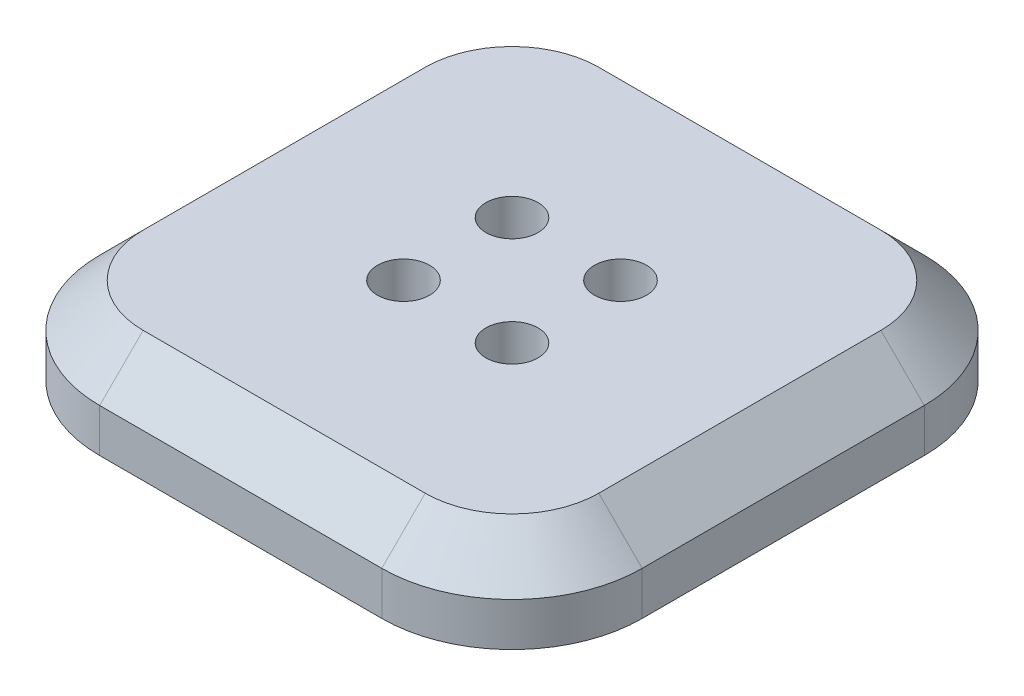
ISO-10303-21;
HEADER;
FILE_DESCRIPTION(('STEP AP214'),'2;1');
FILE_NAME('part.step','',(''),(''),'','','');
FILE_SCHEMA(('AUTOMOTIVE_DESIGN { 1 0 10303 214 1 1 1 1 }'));
ENDSEC;
DATA;
#1=APPLICATION_CONTEXT('core data for automotive mechanical design processes');
#2=APPLICATION_PROTOCOL_DEFINITION('international standard','automotive_design',2000,#1);
#3=PRODUCT_CONTEXT('',#1,'mechanical');
#4=PRODUCT('Part','Part','',(#3));
#5=PRODUCT_RELATED_PRODUCT_CATEGORY('part','',(#4));
#6=PRODUCT_DEFINITION_FORMATION('','',#4);
#7=PRODUCT_DEFINITION_CONTEXT('part definition',#1,'design');
#8=PRODUCT_DEFINITION('design','',#6,#7);
#9=PRODUCT_DEFINITION_SHAPE('','',#8);
#10=(LENGTH_UNIT() NAMED_UNIT(*) SI_UNIT(.MILLI.,.METRE.));
#11=(NAMED_UNIT(*) PLANE_ANGLE_UNIT() SI_UNIT($,.RADIAN.));
#12=(NAMED_UNIT(*) SI_UNIT($,.STERADIAN.) SOLID_ANGLE_UNIT());
#13=UNCERTAINTY_MEASURE_WITH_UNIT(LENGTH_MEASURE(1.E-05),#10,'distance_accuracy_value','');
#14=(GEOMETRIC_REPRESENTATION_CONTEXT(3) GLOBAL_UNCERTAINTY_ASSIGNED_CONTEXT((#13)) GLOBAL_UNIT_ASSIGNED_CONTEXT((#10,
#11,#12)) REPRESENTATION_CONTEXT('',''));
#15=CARTESIAN_POINT('',(0.,0.,0.));
#16=DIRECTION('',(0.,0.,1.));
#17=DIRECTION('',(1.,0.,0.));
#18=AXIS2_PLACEMENT_3D('',#15,#16,#17);
#19=CARTESIAN_POINT('',(62.5,20.,62.5));
#20=DIRECTION('',(-1.,0.,0.));
#21=DIRECTION('',(0.,0.,1.));
#22=AXIS2_PLACEMENT_3D('',#19,#20,#21);
#23=PLANE('',#22);
#24=DIRECTION('',(0.,-1.,0.));
#25=VECTOR('',#24,1.);
#26=CARTESIAN_POINT('',(62.5,20.,-32.5));
#27=LINE('',#26,#25);
#28=CARTESIAN_POINT('',(62.5,0.,-32.5));
#29=VERTEX_POINT('',#28);
#30=CARTESIAN_POINT('',(62.5,9.99999999999996,-32.5));
#31=VERTEX_POINT('',#30);
#32=EDGE_CURVE('E242',#29,#31,#27,.F.);
#33=ORIENTED_EDGE('',*,*,#32,.T.);
#34=DIRECTION('',(0.,0.,1.));
#35=VECTOR('',#34,1.);
#36=CARTESIAN_POINT('',(62.5,9.99999999999996,62.5));
#37=LINE('',#36,#35);
#38=CARTESIAN_POINT('',(62.5,9.99999999999996,32.5));
#39=VERTEX_POINT('',#38);
#40=EDGE_CURVE('E11',#31,#39,#37,.T.);
#41=ORIENTED_EDGE('',*,*,#40,.T.);
#42=DIRECTION('',(0.,-1.,0.));
#43=VECTOR('',#42,1.);
#44=CARTESIAN_POINT('',(62.5,20.,32.5));
#45=LINE('',#44,#43);
#46=CARTESIAN_POINT('',(62.5,0.,32.5));
#47=VERTEX_POINT('',#46);
#48=EDGE_CURVE('E245',#39,#47,#45,.T.);
#49=ORIENTED_EDGE('',*,*,#48,.T.);
#50=DIRECTION('',(0.,0.,-1.));
#51=VECTOR('',#50,1.);
#52=CARTESIAN_POINT('',(62.5,0.,62.5));
#53=LINE('',#52,#51);
#54=EDGE_CURVE('E215',#47,#29,#53,.T.);
#55=ORIENTED_EDGE('',*,*,#54,.T.);
#56=EDGE_LOOP('',(#33,#41,#49,#55));
#57=FACE_BOUND('',#56,.T.);
#58=ADVANCED_FACE('F41',(#57),#23,.F.);
#59=CARTESIAN_POINT('',(-62.5,20.,-62.5));
#60=DIRECTION('',(0.,0.,1.));
#61=DIRECTION('',(1.,0.,0.));
#62=AXIS2_PLACEMENT_3D('',#59,#60,#61);
#63=PLANE('',#62);
#64=DIRECTION('',(0.,-1.,0.));
#65=VECTOR('',#64,1.);
#66=CARTESIAN_POINT('',(-32.5,20.,-62.5));
#67=LINE('',#66,#65);
#68=CARTESIAN_POINT('',(-32.5,0.,-62.5));
#69=VERTEX_POINT('',#68);
#70=CARTESIAN_POINT('',(-32.5,9.99999999999996,-62.5));
#71=VERTEX_POINT('',#70);
#72=EDGE_CURVE('E239',#69,#71,#67,.F.);
#73=ORIENTED_EDGE('',*,*,#72,.T.);
#74=DIRECTION('',(1.,0.,0.));
#75=VECTOR('',#74,1.);
#76=CARTESIAN_POINT('',(-62.5,9.99999999999996,-62.5));
#77=LINE('',#76,#75);
#78=CARTESIAN_POINT('',(32.5,9.99999999999996,-62.5));
#79=VERTEX_POINT('',#78);
#80=EDGE_CURVE('E280',#71,#79,#77,.T.);
#81=ORIENTED_EDGE('',*,*,#80,.T.);
#82=DIRECTION('',(0.,-1.,0.));
#83=VECTOR('',#82,1.);
#84=CARTESIAN_POINT('',(32.5,20.,-62.5));
#85=LINE('',#84,#83);
#86=CARTESIAN_POINT('',(32.5,0.,-62.5));
#87=VERTEX_POINT('',#86);
#88=EDGE_CURVE('E240',#79,#87,#85,.T.);
#89=ORIENTED_EDGE('',*,*,#88,.T.);
#90=DIRECTION('',(-1.,0.,0.));
#91=VECTOR('',#90,1.);
#92=CARTESIAN_POINT('',(-62.5,0.,-62.5));
#93=LINE('',#92,#91);
#94=EDGE_CURVE('E214',#87,#69,#93,.T.);
#95=ORIENTED_EDGE('',*,*,#94,.T.);
#96=EDGE_LOOP('',(#73,#81,#89,#95));
#97=FACE_BOUND('',#96,.T.);
#98=ADVANCED_FACE('F335',(#97),#63,.F.);
#99=CARTESIAN_POINT('',(-62.5,20.,62.5));
#100=DIRECTION('',(1.,0.,0.));
#101=DIRECTION('',(0.,0.,-1.));
#102=AXIS2_PLACEMENT_3D('',#99,#100,#101);
#103=PLANE('',#102);
#104=DIRECTION('',(0.,-1.,0.));
#105=VECTOR('',#104,1.);
#106=CARTESIAN_POINT('',(-62.5,20.,32.5));
#107=LINE('',#106,#105);
#108=CARTESIAN_POINT('',(-62.5,0.,32.5));
#109=VERTEX_POINT('',#108);
#110=CARTESIAN_POINT('',(-62.5,9.99999999999996,32.5));
#111=VERTEX_POINT('',#110);
#112=EDGE_CURVE('E221',#109,#111,#107,.F.);
#113=ORIENTED_EDGE('',*,*,#112,.T.);
#114=DIRECTION('',(0.,0.,-1.));
#115=VECTOR('',#114,1.);
#116=CARTESIAN_POINT('',(-62.5,9.99999999999996,62.5));
#117=LINE('',#116,#115);
#118=CARTESIAN_POINT('',(-62.5,9.99999999999996,-32.5));
#119=VERTEX_POINT('',#118);
#120=EDGE_CURVE('E268',#111,#119,#117,.T.);
#121=ORIENTED_EDGE('',*,*,#120,.T.);
#122=DIRECTION('',(0.,-1.,0.));
#123=VECTOR('',#122,1.);
#124=CARTESIAN_POINT('',(-62.5,20.,-32.5));
#125=LINE('',#124,#123);
#126=CARTESIAN_POINT('',(-62.5,0.,-32.5));
#127=VERTEX_POINT('',#126);
#128=EDGE_CURVE('E230',#119,#127,#125,.T.);
#129=ORIENTED_EDGE('',*,*,#128,.T.);
#130=DIRECTION('',(0.,0.,1.));
#131=VECTOR('',#130,1.);
#132=CARTESIAN_POINT('',(-62.5,0.,62.5));
#133=LINE('',#132,#131);
#134=EDGE_CURVE('E217',#127,#109,#133,.T.);
#135=ORIENTED_EDGE('',*,*,#134,.T.);
#136=EDGE_LOOP('',(#113,#121,#129,#135));
#137=FACE_BOUND('',#136,.T.);
#138=ADVANCED_FACE('F347',(#137),#103,.F.);
#139=CARTESIAN_POINT('',(-62.5,20.,62.5));
#140=DIRECTION('',(0.,0.,-1.));
#141=DIRECTION('',(-1.,0.,0.));
#142=AXIS2_PLACEMENT_3D('',#139,#140,#141);
#143=PLANE('',#142);
#144=DIRECTION('',(0.,-1.,0.));
#145=VECTOR('',#144,1.);
#146=CARTESIAN_POINT('',(32.5,20.,62.5));
#147=LINE('',#146,#145);
#148=CARTESIAN_POINT('',(32.5,0.,62.5));
#149=VERTEX_POINT('',#148);
#150=CARTESIAN_POINT('',(32.5,9.99999999999996,62.5));
#151=VERTEX_POINT('',#150);
#152=EDGE_CURVE('E246',#149,#151,#147,.F.);
#153=ORIENTED_EDGE('',*,*,#152,.T.);
#154=DIRECTION('',(-1.,0.,0.));
#155=VECTOR('',#154,1.);
#156=CARTESIAN_POINT('',(-62.5,9.99999999999996,62.5));
#157=LINE('',#156,#155);
#158=CARTESIAN_POINT('',(-32.5,9.99999999999996,62.5));
#159=VERTEX_POINT('',#158);
#160=EDGE_CURVE('E274',#151,#159,#157,.T.);
#161=ORIENTED_EDGE('',*,*,#160,.T.);
#162=DIRECTION('',(0.,-1.,0.));
#163=VECTOR('',#162,1.);
#164=CARTESIAN_POINT('',(-32.5,20.,62.5));
#165=LINE('',#164,#163);
#166=CARTESIAN_POINT('',(-32.5,0.,62.5));
#167=VERTEX_POINT('',#166);
#168=EDGE_CURVE('E248',#159,#167,#165,.T.);
#169=ORIENTED_EDGE('',*,*,#168,.T.);
#170=DIRECTION('',(1.,0.,0.));
#171=VECTOR('',#170,1.);
#172=CARTESIAN_POINT('',(-62.5,0.,62.5));
#173=LINE('',#172,#171);
#174=EDGE_CURVE('E222',#167,#149,#173,.T.);
#175=ORIENTED_EDGE('',*,*,#174,.T.);
#176=EDGE_LOOP('',(#153,#161,#169,#175));
#177=FACE_BOUND('',#176,.T.);
#178=ADVANCED_FACE('F318',(#177),#143,.F.);
#179=CARTESIAN_POINT('',(0.,20.,0.));
#180=DIRECTION('',(0.,-1.,0.));
#181=DIRECTION('',(0.,0.,-1.));
#182=AXIS2_PLACEMENT_3D('',#179,#180,#181);
#183=PLANE('',#182);
#184=CARTESIAN_POINT('',(-12.5,20.,-12.5));
#185=DIRECTION('',(0.,1.,0.));
#186=DIRECTION('',(0.,0.,1.));
#187=AXIS2_PLACEMENT_3D('',#184,#185,#186);
#188=CIRCLE('',#187,5.99999999999999);
#189=CARTESIAN_POINT('',(-12.5,20.,-6.5));
#190=VERTEX_POINT('',#189);
#191=EDGE_CURVE('E190',#190,#190,#188,.T.);
#192=ORIENTED_EDGE('',*,*,#191,.F.);
#193=EDGE_LOOP('',(#192));
#194=FACE_BOUND('',#193,.T.);
#195=CARTESIAN_POINT('',(12.5,20.,-12.5));
#196=DIRECTION('',(0.,1.,0.));
#197=DIRECTION('',(0.,0.,1.));
#198=AXIS2_PLACEMENT_3D('',#195,#196,#197);
#199=CIRCLE('',#198,5.99999999999999);
#200=CARTESIAN_POINT('',(12.5,20.,-6.5));
#201=VERTEX_POINT('',#200);
#202=EDGE_CURVE('E191',#201,#201,#199,.T.);
#203=ORIENTED_EDGE('',*,*,#202,.F.);
#204=EDGE_LOOP('',(#203));
#205=FACE_BOUND('',#204,.T.);
#206=CARTESIAN_POINT('',(12.5,20.,12.5));
#207=DIRECTION('',(0.,1.,0.));
#208=DIRECTION('',(0.,0.,1.));
#209=AXIS2_PLACEMENT_3D('',#206,#207,#208);
#210=CIRCLE('',#209,5.99999999999999);
#211=CARTESIAN_POINT('',(12.5,20.,18.5));
#212=VERTEX_POINT('',#211);
#213=EDGE_CURVE('E200',#212,#212,#210,.T.);
#214=ORIENTED_EDGE('',*,*,#213,.F.);
#215=EDGE_LOOP('',(#214));
#216=FACE_BOUND('',#215,.T.);
#217=CARTESIAN_POINT('',(-12.5,20.,12.5));
#218=DIRECTION('',(0.,1.,0.));
#219=DIRECTION('',(0.,0.,1.));
#220=AXIS2_PLACEMENT_3D('',#217,#218,#219);
#221=CIRCLE('',#220,5.99999999999999);
#222=CARTESIAN_POINT('',(-12.5,20.,18.5));
#223=VERTEX_POINT('',#222);
#224=EDGE_CURVE('E202',#223,#223,#221,.T.);
#225=ORIENTED_EDGE('',*,*,#224,.F.);
#226=EDGE_LOOP('',(#225));
#227=FACE_BOUND('',#226,.T.);
#228=CARTESIAN_POINT('',(-32.5,20.,-32.5));
#229=DIRECTION('',(0.,-1.,0.));
#230=DIRECTION('',(0.,0.,-1.));
#231=AXIS2_PLACEMENT_3D('',#228,#229,#230);
#232=CIRCLE('',#231,20.);
#233=CARTESIAN_POINT('',(-32.5,20.,-52.5));
#234=VERTEX_POINT('',#233);
#235=CARTESIAN_POINT('',(-52.5,20.,-32.5));
#236=VERTEX_POINT('',#235);
#237=EDGE_CURVE('E261',#234,#236,#232,.F.);
#238=ORIENTED_EDGE('',*,*,#237,.T.);
#239=DIRECTION('',(0.,0.,1.));
#240=VECTOR('',#239,1.);
#241=CARTESIAN_POINT('',(-52.5,20.,0.));
#242=LINE('',#241,#240);
#243=CARTESIAN_POINT('',(-52.5,20.,32.5));
#244=VERTEX_POINT('',#243);
#245=EDGE_CURVE('E264',#236,#244,#242,.T.);
#246=ORIENTED_EDGE('',*,*,#245,.T.);
#247=CARTESIAN_POINT('',(-32.5,20.,32.5));
#248=DIRECTION('',(0.,-1.,0.));
#249=DIRECTION('',(0.,0.,-1.));
#250=AXIS2_PLACEMENT_3D('',#247,#248,#249);
#251=CIRCLE('',#250,20.);
#252=CARTESIAN_POINT('',(-32.5,20.,52.5));
#253=VERTEX_POINT('',#252);
#254=EDGE_CURVE('E263',#244,#253,#251,.F.);
#255=ORIENTED_EDGE('',*,*,#254,.T.);
#256=DIRECTION('',(1.,0.,0.));
#257=VECTOR('',#256,1.);
#258=CARTESIAN_POINT('',(0.,20.,52.5));
#259=LINE('',#258,#257);
#260=CARTESIAN_POINT('',(32.5,20.,52.5));
#261=VERTEX_POINT('',#260);
#262=EDGE_CURVE('E259',#253,#261,#259,.T.);
#263=ORIENTED_EDGE('',*,*,#262,.T.);
#264=CARTESIAN_POINT('',(32.5,20.,32.5));
#265=DIRECTION('',(0.,-1.,0.));
#266=DIRECTION('',(0.,0.,-1.));
#267=AXIS2_PLACEMENT_3D('',#264,#265,#266);
#268=CIRCLE('',#267,20.);
#269=CARTESIAN_POINT('',(52.5,20.,32.5));
#270=VERTEX_POINT('',#269);
#271=EDGE_CURVE('E254',#261,#270,#268,.F.);
#272=ORIENTED_EDGE('',*,*,#271,.T.);
#273=DIRECTION('',(0.,0.,-1.));
#274=VECTOR('',#273,1.);
#275=CARTESIAN_POINT('',(52.5,20.,0.));
#276=LINE('',#275,#274);
#277=CARTESIAN_POINT('',(52.5,20.,-32.5));
#278=VERTEX_POINT('',#277);
#279=EDGE_CURVE('E253',#270,#278,#276,.T.);
#280=ORIENTED_EDGE('',*,*,#279,.T.);
#281=CARTESIAN_POINT('',(32.5,20.,-32.5));
#282=DIRECTION('',(0.,-1.,0.));
#283=DIRECTION('',(0.,0.,-1.));
#284=AXIS2_PLACEMENT_3D('',#281,#282,#283);
#285=CIRCLE('',#284,20.);
#286=CARTESIAN_POINT('',(32.5,20.,-52.5));
#287=VERTEX_POINT('',#286);
#288=EDGE_CURVE('E251',#278,#287,#285,.F.);
#289=ORIENTED_EDGE('',*,*,#288,.T.);
#290=DIRECTION('',(-1.,0.,0.));
#291=VECTOR('',#290,1.);
#292=CARTESIAN_POINT('',(0.,20.,-52.5));
#293=LINE('',#292,#291);
#294=EDGE_CURVE('E260',#287,#234,#293,.T.);
#295=ORIENTED_EDGE('',*,*,#294,.T.);
#296=EDGE_LOOP('',(#238,#246,#255,#263,#272,#280,#289,#295));
#297=FACE_BOUND('',#296,.T.);
#298=ADVANCED_FACE('F356',(#194,#205,#216,#227,#297),#183,.F.);
#299=CARTESIAN_POINT('',(0.,0.,0.));
#300=DIRECTION('',(0.,-1.,0.));
#301=DIRECTION('',(0.,0.,-1.));
#302=AXIS2_PLACEMENT_3D('',#299,#300,#301);
#303=PLANE('',#302);
#304=CARTESIAN_POINT('',(-37.5,0.,37.5));
#305=DIRECTION('',(0.,-1.,0.));
#306=DIRECTION('',(0.,0.,-1.));
#307=AXIS2_PLACEMENT_3D('',#304,#305,#306);
#308=CIRCLE('',#307,5.99999999999998);
#309=CARTESIAN_POINT('',(-37.5,0.,31.5));
#310=VERTEX_POINT('',#309);
#311=EDGE_CURVE('E164',#310,#310,#308,.T.);
#312=ORIENTED_EDGE('',*,*,#311,.F.);
#313=EDGE_LOOP('',(#312));
#314=FACE_BOUND('',#313,.T.);
#315=CARTESIAN_POINT('',(37.5,0.,37.5));
#316=DIRECTION('',(0.,-1.,0.));
#317=DIRECTION('',(0.,0.,-1.));
#318=AXIS2_PLACEMENT_3D('',#315,#316,#317);
#319=CIRCLE('',#318,5.99999999999998);
#320=CARTESIAN_POINT('',(37.5,0.,31.5));
#321=VERTEX_POINT('',#320);
#322=EDGE_CURVE('E163',#321,#321,#319,.T.);
#323=ORIENTED_EDGE('',*,*,#322,.F.);
#324=EDGE_LOOP('',(#323));
#325=FACE_BOUND('',#324,.T.);
#326=CARTESIAN_POINT('',(37.5,0.,-37.5));
#327=DIRECTION('',(0.,-1.,0.));
#328=DIRECTION('',(0.,0.,-1.));
#329=AXIS2_PLACEMENT_3D('',#326,#327,#328);
#330=CIRCLE('',#329,5.99999999999998);
#331=CARTESIAN_POINT('',(37.5,0.,-43.5));
#332=VERTEX_POINT('',#331);
#333=EDGE_CURVE('E174',#332,#332,#330,.T.);
#334=ORIENTED_EDGE('',*,*,#333,.F.);
#335=EDGE_LOOP('',(#334));
#336=FACE_BOUND('',#335,.T.);
#337=CARTESIAN_POINT('',(-37.5,0.,-37.5));
#338=DIRECTION('',(0.,-1.,0.));
#339=DIRECTION('',(0.,0.,-1.));
#340=AXIS2_PLACEMENT_3D('',#337,#338,#339);
#341=CIRCLE('',#340,5.99999999999998);
#342=CARTESIAN_POINT('',(-37.5,0.,-43.5));
#343=VERTEX_POINT('',#342);
#344=EDGE_CURVE('E182',#343,#343,#341,.T.);
#345=ORIENTED_EDGE('',*,*,#344,.F.);
#346=EDGE_LOOP('',(#345));
#347=FACE_BOUND('',#346,.T.);
#348=ORIENTED_EDGE('',*,*,#134,.F.);
#349=CARTESIAN_POINT('',(-32.5,0.,-32.5));
#350=DIRECTION('',(0.,-1.,0.));
#351=DIRECTION('',(0.,0.,-1.));
#352=AXIS2_PLACEMENT_3D('',#349,#350,#351);
#353=CIRCLE('',#352,30.);
#354=EDGE_CURVE('E232',#127,#69,#353,.T.);
#355=ORIENTED_EDGE('',*,*,#354,.T.);
#356=ORIENTED_EDGE('',*,*,#94,.F.);
#357=CARTESIAN_POINT('',(32.5,0.,-32.5));
#358=DIRECTION('',(0.,-1.,0.));
#359=DIRECTION('',(0.,0.,-1.));
#360=AXIS2_PLACEMENT_3D('',#357,#358,#359);
#361=CIRCLE('',#360,30.);
#362=EDGE_CURVE('E231',#87,#29,#361,.T.);
#363=ORIENTED_EDGE('',*,*,#362,.T.);
#364=ORIENTED_EDGE('',*,*,#54,.F.);
#365=CARTESIAN_POINT('',(32.5,0.,32.5));
#366=DIRECTION('',(0.,-1.,0.));
#367=DIRECTION('',(0.,0.,-1.));
#368=AXIS2_PLACEMENT_3D('',#365,#366,#367);
#369=CIRCLE('',#368,30.);
#370=EDGE_CURVE('E233',#47,#149,#369,.T.);
#371=ORIENTED_EDGE('',*,*,#370,.T.);
#372=ORIENTED_EDGE('',*,*,#174,.F.);
#373=CARTESIAN_POINT('',(-32.5,0.,32.5));
#374=DIRECTION('',(0.,-1.,0.));
#375=DIRECTION('',(0.,0.,-1.));
#376=AXIS2_PLACEMENT_3D('',#373,#374,#375);
#377=CIRCLE('',#376,30.);
#378=EDGE_CURVE('E227',#167,#109,#377,.T.);
#379=ORIENTED_EDGE('',*,*,#378,.T.);
#380=EDGE_LOOP('',(#348,#355,#356,#363,#364,#371,#372,#379));
#381=FACE_BOUND('',#380,.T.);
#382=ADVANCED_FACE('F322',(#314,#325,#336,#347,#381),#303,.T.);
#383=CARTESIAN_POINT('',(-32.5,20.,-32.5));
#384=DIRECTION('',(0.,-1.,0.));
#385=DIRECTION('',(0.,0.,-1.));
#386=AXIS2_PLACEMENT_3D('',#383,#384,#385);
#387=CYLINDRICAL_SURFACE('',#386,30.);
#388=ORIENTED_EDGE('',*,*,#128,.F.);
#389=CARTESIAN_POINT('',(-32.5,9.99999999999996,-32.5));
#390=DIRECTION('',(0.,-1.,0.));
#391=DIRECTION('',(0.,0.,-1.));
#392=AXIS2_PLACEMENT_3D('',#389,#390,#391);
#393=CIRCLE('',#392,30.);
#394=EDGE_CURVE('E272',#119,#71,#393,.T.);
#395=ORIENTED_EDGE('',*,*,#394,.T.);
#396=ORIENTED_EDGE('',*,*,#72,.F.);
#397=ORIENTED_EDGE('',*,*,#354,.F.);
#398=EDGE_LOOP('',(#388,#395,#396,#397));
#399=FACE_BOUND('',#398,.T.);
#400=ADVANCED_FACE('F338',(#399),#387,.T.);
#401=CARTESIAN_POINT('',(32.5,20.,-32.5));
#402=DIRECTION('',(0.,-1.,0.));
#403=DIRECTION('',(0.,0.,-1.));
#404=AXIS2_PLACEMENT_3D('',#401,#402,#403);
#405=CYLINDRICAL_SURFACE('',#404,30.);
#406=ORIENTED_EDGE('',*,*,#88,.F.);
#407=CARTESIAN_POINT('',(32.5,9.99999999999996,-32.5));
#408=DIRECTION('',(0.,-1.,0.));
#409=DIRECTION('',(0.,0.,-1.));
#410=AXIS2_PLACEMENT_3D('',#407,#408,#409);
#411=CIRCLE('',#410,30.);
#412=EDGE_CURVE('E51',#79,#31,#411,.T.);
#413=ORIENTED_EDGE('',*,*,#412,.T.);
#414=ORIENTED_EDGE('',*,*,#32,.F.);
#415=ORIENTED_EDGE('',*,*,#362,.F.);
#416=EDGE_LOOP('',(#406,#413,#414,#415));
#417=FACE_BOUND('',#416,.T.);
#418=ADVANCED_FACE('F327',(#417),#405,.T.);
#419=CARTESIAN_POINT('',(32.5,20.,32.5));
#420=DIRECTION('',(0.,-1.,0.));
#421=DIRECTION('',(0.,0.,-1.));
#422=AXIS2_PLACEMENT_3D('',#419,#420,#421);
#423=CYLINDRICAL_SURFACE('',#422,30.);
#424=ORIENTED_EDGE('',*,*,#48,.F.);
#425=CARTESIAN_POINT('',(32.5,9.99999999999996,32.5));
#426=DIRECTION('',(0.,-1.,0.));
#427=DIRECTION('',(0.,0.,-1.));
#428=AXIS2_PLACEMENT_3D('',#425,#426,#427);
#429=CIRCLE('',#428,30.);
#430=EDGE_CURVE('E276',#39,#151,#429,.T.);
#431=ORIENTED_EDGE('',*,*,#430,.T.);
#432=ORIENTED_EDGE('',*,*,#152,.F.);
#433=ORIENTED_EDGE('',*,*,#370,.F.);
#434=EDGE_LOOP('',(#424,#431,#432,#433));
#435=FACE_BOUND('',#434,.T.);
#436=ADVANCED_FACE('F312',(#435),#423,.T.);
#437=CARTESIAN_POINT('',(-32.5,20.,32.5));
#438=DIRECTION('',(0.,-1.,0.));
#439=DIRECTION('',(0.,0.,-1.));
#440=AXIS2_PLACEMENT_3D('',#437,#438,#439);
#441=CYLINDRICAL_SURFACE('',#440,30.);
#442=ORIENTED_EDGE('',*,*,#168,.F.);
#443=CARTESIAN_POINT('',(-32.5,9.99999999999996,32.5));
#444=DIRECTION('',(0.,-1.,0.));
#445=DIRECTION('',(0.,0.,-1.));
#446=AXIS2_PLACEMENT_3D('',#443,#444,#445);
#447=CIRCLE('',#446,30.);
#448=EDGE_CURVE('E271',#159,#111,#447,.T.);
#449=ORIENTED_EDGE('',*,*,#448,.T.);
#450=ORIENTED_EDGE('',*,*,#112,.F.);
#451=ORIENTED_EDGE('',*,*,#378,.F.);
#452=EDGE_LOOP('',(#442,#449,#450,#451));
#453=FACE_BOUND('',#452,.T.);
#454=ADVANCED_FACE('F390',(#453),#441,.T.);
#455=CARTESIAN_POINT('',(52.5,20.,0.));
#456=DIRECTION('',(-0.707106781186549,-0.707106781186547,0.));
#457=DIRECTION('',(0.,0.,-1.));
#458=AXIS2_PLACEMENT_3D('',#455,#456,#457);
#459=PLANE('',#458);
#460=DIRECTION('',(-0.707106781186547,0.707106781186549,0.));
#461=VECTOR('',#460,1.);
#462=CARTESIAN_POINT('',(62.5,9.99999999999996,32.5));
#463=LINE('',#462,#461);
#464=EDGE_CURVE('E298',#39,#270,#463,.T.);
#465=ORIENTED_EDGE('',*,*,#464,.F.);
#466=ORIENTED_EDGE('',*,*,#40,.F.);
#467=DIRECTION('',(0.707106781186547,-0.707106781186549,0.));
#468=VECTOR('',#467,1.);
#469=CARTESIAN_POINT('',(52.5,20.,-32.5));
#470=LINE('',#469,#468);
#471=EDGE_CURVE('E46',#278,#31,#470,.T.);
#472=ORIENTED_EDGE('',*,*,#471,.F.);
#473=ORIENTED_EDGE('',*,*,#279,.F.);
#474=EDGE_LOOP('',(#465,#466,#472,#473));
#475=FACE_BOUND('',#474,.T.);
#476=ADVANCED_FACE('F42',(#475),#459,.F.);
#477=CARTESIAN_POINT('',(32.5,20.,-32.5));
#478=DIRECTION('',(0.,-1.,0.));
#479=DIRECTION('',(0.,0.,-1.));
#480=AXIS2_PLACEMENT_3D('',#477,#478,#479);
#481=CONICAL_SURFACE('',#480,20.,0.785398163397447);
#482=ORIENTED_EDGE('',*,*,#471,.T.);
#483=ORIENTED_EDGE('',*,*,#412,.F.);
#484=DIRECTION('',(0.,-0.707106781186549,-0.707106781186547));
#485=VECTOR('',#484,1.);
#486=CARTESIAN_POINT('',(32.5,20.,-52.5));
#487=LINE('',#486,#485);
#488=EDGE_CURVE('E294',#287,#79,#487,.T.);
#489=ORIENTED_EDGE('',*,*,#488,.F.);
#490=ORIENTED_EDGE('',*,*,#288,.F.);
#491=EDGE_LOOP('',(#482,#483,#489,#490));
#492=FACE_BOUND('',#491,.T.);
#493=ADVANCED_FACE('F308',(#492),#481,.T.);
#494=CARTESIAN_POINT('',(32.5,20.,32.5));
#495=DIRECTION('',(0.,-1.,0.));
#496=DIRECTION('',(0.,0.,-1.));
#497=AXIS2_PLACEMENT_3D('',#494,#495,#496);
#498=CONICAL_SURFACE('',#497,20.,0.785398163397447);
#499=ORIENTED_EDGE('',*,*,#464,.T.);
#500=ORIENTED_EDGE('',*,*,#271,.F.);
#501=DIRECTION('',(0.,0.707106781186549,-0.707106781186547));
#502=VECTOR('',#501,1.);
#503=CARTESIAN_POINT('',(32.5,9.99999999999996,62.5));
#504=LINE('',#503,#502);
#505=EDGE_CURVE('E292',#151,#261,#504,.T.);
#506=ORIENTED_EDGE('',*,*,#505,.F.);
#507=ORIENTED_EDGE('',*,*,#430,.F.);
#508=EDGE_LOOP('',(#499,#500,#506,#507));
#509=FACE_BOUND('',#508,.T.);
#510=ADVANCED_FACE('F313',(#509),#498,.T.);
#511=CARTESIAN_POINT('',(0.,20.,-52.5));
#512=DIRECTION('',(0.,-0.707106781186547,0.707106781186549));
#513=DIRECTION('',(-1.,0.,0.));
#514=AXIS2_PLACEMENT_3D('',#511,#512,#513);
#515=PLANE('',#514);
#516=ORIENTED_EDGE('',*,*,#488,.T.);
#517=ORIENTED_EDGE('',*,*,#80,.F.);
#518=DIRECTION('',(0.,-0.707106781186549,-0.707106781186547));
#519=VECTOR('',#518,1.);
#520=CARTESIAN_POINT('',(-32.5,20.,-52.5));
#521=LINE('',#520,#519);
#522=EDGE_CURVE('E286',#234,#71,#521,.T.);
#523=ORIENTED_EDGE('',*,*,#522,.F.);
#524=ORIENTED_EDGE('',*,*,#294,.F.);
#525=EDGE_LOOP('',(#516,#517,#523,#524));
#526=FACE_BOUND('',#525,.T.);
#527=ADVANCED_FACE('F363',(#526),#515,.F.);
#528=CARTESIAN_POINT('',(0.,20.,52.5));
#529=DIRECTION('',(0.,-0.707106781186547,-0.707106781186549));
#530=DIRECTION('',(1.,0.,0.));
#531=AXIS2_PLACEMENT_3D('',#528,#529,#530);
#532=PLANE('',#531);
#533=ORIENTED_EDGE('',*,*,#505,.T.);
#534=ORIENTED_EDGE('',*,*,#262,.F.);
#535=DIRECTION('',(0.,0.707106781186549,-0.707106781186547));
#536=VECTOR('',#535,1.);
#537=CARTESIAN_POINT('',(-32.5,9.99999999999996,62.5));
#538=LINE('',#537,#536);
#539=EDGE_CURVE('E284',#159,#253,#538,.T.);
#540=ORIENTED_EDGE('',*,*,#539,.F.);
#541=ORIENTED_EDGE('',*,*,#160,.F.);
#542=EDGE_LOOP('',(#533,#534,#540,#541));
#543=FACE_BOUND('',#542,.T.);
#544=ADVANCED_FACE('F361',(#543),#532,.F.);
#545=CARTESIAN_POINT('',(-32.5,20.,-32.5));
#546=DIRECTION('',(0.,-1.,0.));
#547=DIRECTION('',(0.,0.,-1.));
#548=AXIS2_PLACEMENT_3D('',#545,#546,#547);
#549=CONICAL_SURFACE('',#548,20.,0.785398163397447);
#550=ORIENTED_EDGE('',*,*,#522,.T.);
#551=ORIENTED_EDGE('',*,*,#394,.F.);
#552=DIRECTION('',(-0.707106781186547,-0.707106781186549,0.));
#553=VECTOR('',#552,1.);
#554=CARTESIAN_POINT('',(-52.5,20.,-32.5));
#555=LINE('',#554,#553);
#556=EDGE_CURVE('E281',#236,#119,#555,.T.);
#557=ORIENTED_EDGE('',*,*,#556,.F.);
#558=ORIENTED_EDGE('',*,*,#237,.F.);
#559=EDGE_LOOP('',(#550,#551,#557,#558));
#560=FACE_BOUND('',#559,.T.);
#561=ADVANCED_FACE('F339',(#560),#549,.T.);
#562=CARTESIAN_POINT('',(-32.5,20.,32.5));
#563=DIRECTION('',(0.,-1.,0.));
#564=DIRECTION('',(0.,0.,-1.));
#565=AXIS2_PLACEMENT_3D('',#562,#563,#564);
#566=CONICAL_SURFACE('',#565,20.,0.785398163397447);
#567=ORIENTED_EDGE('',*,*,#539,.T.);
#568=ORIENTED_EDGE('',*,*,#254,.F.);
#569=DIRECTION('',(0.707106781186547,0.707106781186549,0.));
#570=VECTOR('',#569,1.);
#571=CARTESIAN_POINT('',(-62.5,9.99999999999996,32.5));
#572=LINE('',#571,#570);
#573=EDGE_CURVE('E211',#111,#244,#572,.T.);
#574=ORIENTED_EDGE('',*,*,#573,.F.);
#575=ORIENTED_EDGE('',*,*,#448,.F.);
#576=EDGE_LOOP('',(#567,#568,#574,#575));
#577=FACE_BOUND('',#576,.T.);
#578=ADVANCED_FACE('F352',(#577),#566,.T.);
#579=CARTESIAN_POINT('',(-52.5,20.,0.));
#580=DIRECTION('',(0.707106781186549,-0.707106781186547,0.));
#581=DIRECTION('',(0.,0.,1.));
#582=AXIS2_PLACEMENT_3D('',#579,#580,#581);
#583=PLANE('',#582);
#584=ORIENTED_EDGE('',*,*,#556,.T.);
#585=ORIENTED_EDGE('',*,*,#120,.F.);
#586=ORIENTED_EDGE('',*,*,#573,.T.);
#587=ORIENTED_EDGE('',*,*,#245,.F.);
#588=EDGE_LOOP('',(#584,#585,#586,#587));
#589=FACE_BOUND('',#588,.T.);
#590=ADVANCED_FACE('F348',(#589),#583,.F.);
#591=CARTESIAN_POINT('',(-12.5,10.,12.5));
#592=DIRECTION('',(0.,1.,0.));
#593=DIRECTION('',(0.,0.,1.));
#594=AXIS2_PLACEMENT_3D('',#591,#592,#593);
#595=CONICAL_SURFACE('',#594,5.99999999999999,1.02974425867665);
#596=CARTESIAN_POINT('',(-12.5,6.39483628583465,12.5));
#597=VERTEX_POINT('',#596);
#598=VERTEX_LOOP('',#597);
#599=FACE_BOUND('',#598,.T.);
#600=CARTESIAN_POINT('',(-12.5,10.,12.5));
#601=DIRECTION('',(0.,1.,0.));
#602=DIRECTION('',(0.,0.,1.));
#603=AXIS2_PLACEMENT_3D('',#600,#601,#602);
#604=CIRCLE('',#603,5.99999999999999);
#605=CARTESIAN_POINT('',(-12.5,10.,18.5));
#606=VERTEX_POINT('',#605);
#607=EDGE_CURVE('E208',#606,#606,#604,.T.);
#608=ORIENTED_EDGE('',*,*,#607,.T.);
#609=EDGE_LOOP('',(#608));
#610=FACE_BOUND('',#609,.T.);
#611=ADVANCED_FACE('F400',(#599,#610),#595,.F.);
#612=CARTESIAN_POINT('',(-12.5,20.,12.5));
#613=DIRECTION('',(0.,1.,0.));
#614=DIRECTION('',(0.,0.,1.));
#615=AXIS2_PLACEMENT_3D('',#612,#613,#614);
#616=CYLINDRICAL_SURFACE('',#615,5.99999999999999);
#617=ORIENTED_EDGE('',*,*,#607,.F.);
#618=EDGE_LOOP('',(#617));
#619=FACE_BOUND('',#618,.T.);
#620=ORIENTED_EDGE('',*,*,#224,.T.);
#621=EDGE_LOOP('',(#620));
#622=FACE_BOUND('',#621,.T.);
#623=ADVANCED_FACE('F535',(#619,#622),#616,.F.);
#624=CARTESIAN_POINT('',(12.5,10.,12.5));
#625=DIRECTION('',(0.,1.,0.));
#626=DIRECTION('',(0.,0.,1.));
#627=AXIS2_PLACEMENT_3D('',#624,#625,#626);
#628=CONICAL_SURFACE('',#627,5.99999999999999,1.02974425867665);
#629=CARTESIAN_POINT('',(12.5,6.39483628583465,12.5));
#630=VERTEX_POINT('',#629);
#631=VERTEX_LOOP('',#630);
#632=FACE_BOUND('',#631,.T.);
#633=CARTESIAN_POINT('',(12.5,10.,12.5));
#634=DIRECTION('',(0.,1.,0.));
#635=DIRECTION('',(0.,0.,1.));
#636=AXIS2_PLACEMENT_3D('',#633,#634,#635);
#637=CIRCLE('',#636,5.99999999999999);
#638=CARTESIAN_POINT('',(12.5,10.,18.5));
#639=VERTEX_POINT('',#638);
#640=EDGE_CURVE('E205',#639,#639,#637,.T.);
#641=ORIENTED_EDGE('',*,*,#640,.T.);
#642=EDGE_LOOP('',(#641));
#643=FACE_BOUND('',#642,.T.);
#644=ADVANCED_FACE('F541',(#632,#643),#628,.F.);
#645=CARTESIAN_POINT('',(12.5,20.,12.5));
#646=DIRECTION('',(0.,1.,0.));
#647=DIRECTION('',(0.,0.,1.));
#648=AXIS2_PLACEMENT_3D('',#645,#646,#647);
#649=CYLINDRICAL_SURFACE('',#648,5.99999999999999);
#650=ORIENTED_EDGE('',*,*,#640,.F.);
#651=EDGE_LOOP('',(#650));
#652=FACE_BOUND('',#651,.T.);
#653=ORIENTED_EDGE('',*,*,#213,.T.);
#654=EDGE_LOOP('',(#653));
#655=FACE_BOUND('',#654,.T.);
#656=ADVANCED_FACE('F549',(#652,#655),#649,.F.);
#657=CARTESIAN_POINT('',(12.5,10.,-12.5));
#658=DIRECTION('',(0.,1.,0.));
#659=DIRECTION('',(0.,0.,1.));
#660=AXIS2_PLACEMENT_3D('',#657,#658,#659);
#661=CONICAL_SURFACE('',#660,5.99999999999999,1.02974425867665);
#662=CARTESIAN_POINT('',(12.5,6.39483628583465,-12.5));
#663=VERTEX_POINT('',#662);
#664=VERTEX_LOOP('',#663);
#665=FACE_BOUND('',#664,.T.);
#666=CARTESIAN_POINT('',(12.5,10.,-12.5));
#667=DIRECTION('',(0.,1.,0.));
#668=DIRECTION('',(0.,0.,1.));
#669=AXIS2_PLACEMENT_3D('',#666,#667,#668);
#670=CIRCLE('',#669,5.99999999999999);
#671=CARTESIAN_POINT('',(12.5,10.,-6.5));
#672=VERTEX_POINT('',#671);
#673=EDGE_CURVE('E198',#672,#672,#670,.T.);
#674=ORIENTED_EDGE('',*,*,#673,.T.);
#675=EDGE_LOOP('',(#674));
#676=FACE_BOUND('',#675,.T.);
#677=ADVANCED_FACE('F557',(#665,#676),#661,.F.);
#678=CARTESIAN_POINT('',(12.5,20.,-12.5));
#679=DIRECTION('',(0.,1.,0.));
#680=DIRECTION('',(0.,0.,1.));
#681=AXIS2_PLACEMENT_3D('',#678,#679,#680);
#682=CYLINDRICAL_SURFACE('',#681,5.99999999999999);
#683=ORIENTED_EDGE('',*,*,#673,.F.);
#684=EDGE_LOOP('',(#683));
#685=FACE_BOUND('',#684,.T.);
#686=ORIENTED_EDGE('',*,*,#202,.T.);
#687=EDGE_LOOP('',(#686));
#688=FACE_BOUND('',#687,.T.);
#689=ADVANCED_FACE('F566',(#685,#688),#682,.F.);
#690=CARTESIAN_POINT('',(-12.5,10.,-12.5));
#691=DIRECTION('',(0.,1.,0.));
#692=DIRECTION('',(0.,0.,1.));
#693=AXIS2_PLACEMENT_3D('',#690,#691,#692);
#694=CONICAL_SURFACE('',#693,5.99999999999999,1.02974425867665);
#695=CARTESIAN_POINT('',(-12.5,6.39483628583465,-12.5));
#696=VERTEX_POINT('',#695);
#697=VERTEX_LOOP('',#696);
#698=FACE_BOUND('',#697,.T.);
#699=CARTESIAN_POINT('',(-12.5,10.,-12.5));
#700=DIRECTION('',(0.,1.,0.));
#701=DIRECTION('',(0.,0.,1.));
#702=AXIS2_PLACEMENT_3D('',#699,#700,#701);
#703=CIRCLE('',#702,5.99999999999999);
#704=CARTESIAN_POINT('',(-12.5,10.,-6.5));
#705=VERTEX_POINT('',#704);
#706=EDGE_CURVE('E189',#705,#705,#703,.T.);
#707=ORIENTED_EDGE('',*,*,#706,.T.);
#708=EDGE_LOOP('',(#707));
#709=FACE_BOUND('',#708,.T.);
#710=ADVANCED_FACE('F580',(#698,#709),#694,.F.);
#711=CARTESIAN_POINT('',(-12.5,20.,-12.5));
#712=DIRECTION('',(0.,1.,0.));
#713=DIRECTION('',(0.,0.,1.));
#714=AXIS2_PLACEMENT_3D('',#711,#712,#713);
#715=CYLINDRICAL_SURFACE('',#714,5.99999999999999);
#716=ORIENTED_EDGE('',*,*,#706,.F.);
#717=EDGE_LOOP('',(#716));
#718=FACE_BOUND('',#717,.T.);
#719=ORIENTED_EDGE('',*,*,#191,.T.);
#720=EDGE_LOOP('',(#719));
#721=FACE_BOUND('',#720,.T.);
#722=ADVANCED_FACE('F588',(#718,#721),#715,.F.);
#723=CARTESIAN_POINT('',(-37.5,9.99999999999999,-37.5));
#724=DIRECTION('',(0.,-1.,0.));
#725=DIRECTION('',(0.,0.,-1.));
#726=AXIS2_PLACEMENT_3D('',#723,#724,#725);
#727=CONICAL_SURFACE('',#726,5.99999999999998,1.02974425867665);
#728=CARTESIAN_POINT('',(-37.5,13.6051637141654,-37.5));
#729=VERTEX_POINT('',#728);
#730=VERTEX_LOOP('',#729);
#731=FACE_BOUND('',#730,.T.);
#732=CARTESIAN_POINT('',(-37.5,9.99999999999999,-37.5));
#733=DIRECTION('',(0.,-1.,0.));
#734=DIRECTION('',(0.,0.,-1.));
#735=AXIS2_PLACEMENT_3D('',#732,#733,#734);
#736=CIRCLE('',#735,5.99999999999998);
#737=CARTESIAN_POINT('',(-37.5,9.99999999999999,-43.5));
#738=VERTEX_POINT('',#737);
#739=EDGE_CURVE('E184',#738,#738,#736,.T.);
#740=ORIENTED_EDGE('',*,*,#739,.T.);
#741=EDGE_LOOP('',(#740));
#742=FACE_BOUND('',#741,.T.);
#743=ADVANCED_FACE('F594',(#731,#742),#727,.F.);
#744=CARTESIAN_POINT('',(-37.5,0.,-37.5));
#745=DIRECTION('',(0.,-1.,0.));
#746=DIRECTION('',(0.,0.,-1.));
#747=AXIS2_PLACEMENT_3D('',#744,#745,#746);
#748=CYLINDRICAL_SURFACE('',#747,5.99999999999998);
#749=ORIENTED_EDGE('',*,*,#739,.F.);
#750=EDGE_LOOP('',(#749));
#751=FACE_BOUND('',#750,.T.);
#752=ORIENTED_EDGE('',*,*,#344,.T.);
#753=EDGE_LOOP('',(#752));
#754=FACE_BOUND('',#753,.T.);
#755=ADVANCED_FACE('F603',(#751,#754),#748,.F.);
#756=CARTESIAN_POINT('',(37.5,9.99999999999999,-37.5));
#757=DIRECTION('',(0.,-1.,0.));
#758=DIRECTION('',(0.,0.,-1.));
#759=AXIS2_PLACEMENT_3D('',#756,#757,#758);
#760=CONICAL_SURFACE('',#759,5.99999999999998,1.02974425867665);
#761=CARTESIAN_POINT('',(37.5,13.6051637141654,-37.5));
#762=VERTEX_POINT('',#761);
#763=VERTEX_LOOP('',#762);
#764=FACE_BOUND('',#763,.T.);
#765=CARTESIAN_POINT('',(37.5,9.99999999999999,-37.5));
#766=DIRECTION('',(0.,-1.,0.));
#767=DIRECTION('',(0.,0.,-1.));
#768=AXIS2_PLACEMENT_3D('',#765,#766,#767);
#769=CIRCLE('',#768,5.99999999999998);
#770=CARTESIAN_POINT('',(37.5,9.99999999999999,-43.5));
#771=VERTEX_POINT('',#770);
#772=EDGE_CURVE('E176',#771,#771,#769,.T.);
#773=ORIENTED_EDGE('',*,*,#772,.T.);
#774=EDGE_LOOP('',(#773));
#775=FACE_BOUND('',#774,.T.);
#776=ADVANCED_FACE('F611',(#764,#775),#760,.F.);
#777=CARTESIAN_POINT('',(37.5,0.,-37.5));
#778=DIRECTION('',(0.,-1.,0.));
#779=DIRECTION('',(0.,0.,-1.));
#780=AXIS2_PLACEMENT_3D('',#777,#778,#779);
#781=CYLINDRICAL_SURFACE('',#780,5.99999999999998);
#782=ORIENTED_EDGE('',*,*,#772,.F.);
#783=EDGE_LOOP('',(#782));
#784=FACE_BOUND('',#783,.T.);
#785=ORIENTED_EDGE('',*,*,#333,.T.);
#786=EDGE_LOOP('',(#785));
#787=FACE_BOUND('',#786,.T.);
#788=ADVANCED_FACE('F625',(#784,#787),#781,.F.);
#789=CARTESIAN_POINT('',(37.5,9.99999999999999,37.5));
#790=DIRECTION('',(0.,-1.,0.));
#791=DIRECTION('',(0.,0.,-1.));
#792=AXIS2_PLACEMENT_3D('',#789,#790,#791);
#793=CONICAL_SURFACE('',#792,5.99999999999998,1.02974425867665);
#794=CARTESIAN_POINT('',(37.5,13.6051637141654,37.5));
#795=VERTEX_POINT('',#794);
#796=VERTEX_LOOP('',#795);
#797=FACE_BOUND('',#796,.T.);
#798=CARTESIAN_POINT('',(37.5,9.99999999999999,37.5));
#799=DIRECTION('',(0.,-1.,0.));
#800=DIRECTION('',(0.,0.,-1.));
#801=AXIS2_PLACEMENT_3D('',#798,#799,#800);
#802=CIRCLE('',#801,5.99999999999998);
#803=CARTESIAN_POINT('',(37.5,9.99999999999999,31.5));
#804=VERTEX_POINT('',#803);
#805=EDGE_CURVE('E169',#804,#804,#802,.T.);
#806=ORIENTED_EDGE('',*,*,#805,.T.);
#807=EDGE_LOOP('',(#806));
#808=FACE_BOUND('',#807,.T.);
#809=ADVANCED_FACE('F633',(#797,#808),#793,.F.);
#810=CARTESIAN_POINT('',(37.5,0.,37.5));
#811=DIRECTION('',(0.,-1.,0.));
#812=DIRECTION('',(0.,0.,-1.));
#813=AXIS2_PLACEMENT_3D('',#810,#811,#812);
#814=CYLINDRICAL_SURFACE('',#813,5.99999999999998);
#815=ORIENTED_EDGE('',*,*,#805,.F.);
#816=EDGE_LOOP('',(#815));
#817=FACE_BOUND('',#816,.T.);
#818=ORIENTED_EDGE('',*,*,#322,.T.);
#819=EDGE_LOOP('',(#818));
#820=FACE_BOUND('',#819,.T.);
#821=ADVANCED_FACE('F158',(#817,#820),#814,.F.);
#822=CARTESIAN_POINT('',(-37.5,9.99999999999999,37.5));
#823=DIRECTION('',(0.,-1.,0.));
#824=DIRECTION('',(0.,0.,-1.));
#825=AXIS2_PLACEMENT_3D('',#822,#823,#824);
#826=CONICAL_SURFACE('',#825,5.99999999999998,1.02974425867665);
#827=CARTESIAN_POINT('',(-37.5,13.6051637141654,37.5));
#828=VERTEX_POINT('',#827);
#829=VERTEX_LOOP('',#828);
#830=FACE_BOUND('',#829,.T.);
#831=CARTESIAN_POINT('',(-37.5,9.99999999999999,37.5));
#832=DIRECTION('',(0.,-1.,0.));
#833=DIRECTION('',(0.,0.,-1.));
#834=AXIS2_PLACEMENT_3D('',#831,#832,#833);
#835=CIRCLE('',#834,5.99999999999998);
#836=CARTESIAN_POINT('',(-37.5,9.99999999999999,31.5));
#837=VERTEX_POINT('',#836);
#838=EDGE_CURVE('E165',#837,#837,#835,.T.);
#839=ORIENTED_EDGE('',*,*,#838,.T.);
#840=EDGE_LOOP('',(#839));
#841=FACE_BOUND('',#840,.T.);
#842=ADVANCED_FACE('F152',(#830,#841),#826,.F.);
#843=CARTESIAN_POINT('',(-37.5,0.,37.5));
#844=DIRECTION('',(0.,-1.,0.));
#845=DIRECTION('',(0.,0.,-1.));
#846=AXIS2_PLACEMENT_3D('',#843,#844,#845);
#847=CYLINDRICAL_SURFACE('',#846,5.99999999999998);
#848=ORIENTED_EDGE('',*,*,#838,.F.);
#849=EDGE_LOOP('',(#848));
#850=FACE_BOUND('',#849,.T.);
#851=ORIENTED_EDGE('',*,*,#311,.T.);
#852=EDGE_LOOP('',(#851));
#853=FACE_BOUND('',#852,.T.);
#854=ADVANCED_FACE('F160',(#850,#853),#847,.F.);
#855=CLOSED_SHELL('',(#58,#98,#138,#178,#298,#382,#400,#418,#436,#454,#476,#493,#510,#527,#544,
#561,#578,#590,#611,#623,#644,#656,#677,#689,#710,#722,#743,#755,#776,#788,#809,#821,#842,#854));
#856=MANIFOLD_SOLID_BREP('B2',#855);
#857=ADVANCED_BREP_SHAPE_REPRESENTATION('',(#18,#856),#14);
#858=SHAPE_DEFINITION_REPRESENTATION(#9,#857);
ENDSEC;
END-ISO-10303-21;
